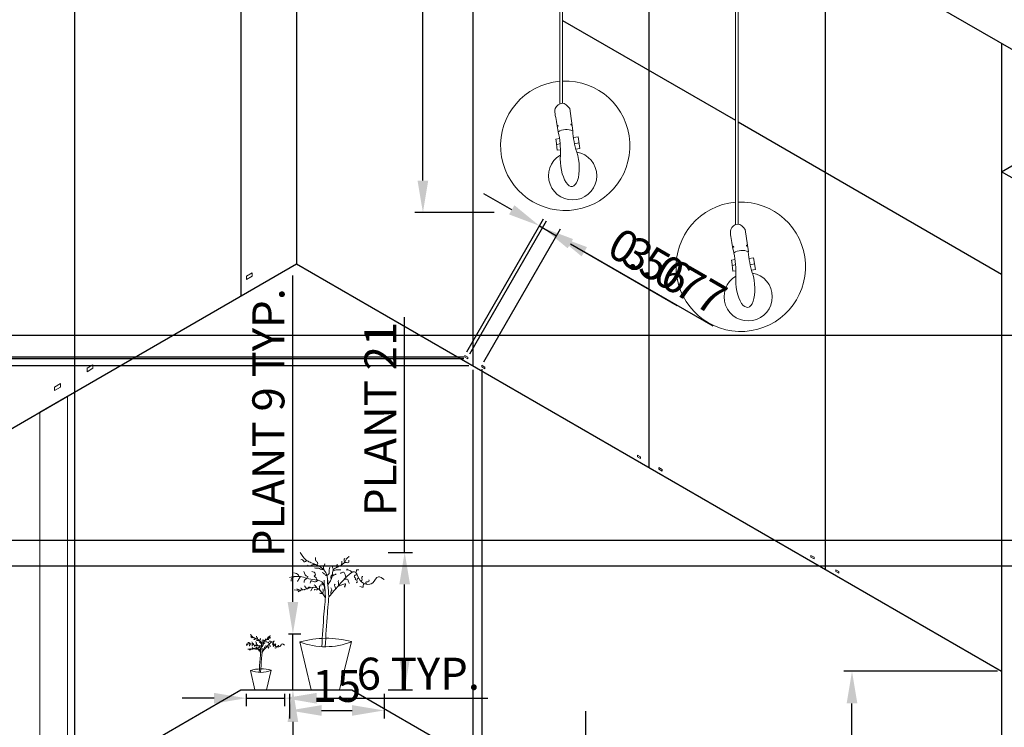
# Model space of a CAD drawing. Units: centimetres. Extents: x 2148 to 2649, y 4226 to 4785.
# Tile 4 of 6: x 2402 to 2555, y 4539 to 4649. Entities that reach past the tile are written whole.
import ezdxf

# ---------------------------------------------------------------- set-up
doc = ezdxf.new("R2010")
doc.units = ezdxf.units.CM
for name, color, linetype, lineweight in [('A-ANNO-DIMS', 63, 'Continuous', 18), ('A-ANNO-REFR', 8, 'Continuous', 13), ('A-FLOR-BSPL', 21, 'Continuous', 13), ('A-FLOR-CASE', 21, 'Continuous', 25), ('A-FLOR-CASE-HDW', 21, 'Continuous', 18), ('A-FLOR-CASE-TALL', 30, 'Continuous', 30), ('A-FLOR-CTOP', 21, 'Continuous', 25), ('E-LITE', 21, 'Continuous', 18), ('TREES', 80, 'Continuous', 13)]:
    doc.layers.add(name, color=color, linetype=linetype, lineweight=lineweight)
doc.styles.get("Standard").update_dxf_attribs({"font": 'arial.ttf'})
doc.dimstyles.new('ISO-25', dxfattribs={"dimtxt": 5, "dimasz": 5, "dimexe": 1.25, "dimexo": 0.625, "dimtad": 1, "dimdec": 1, "dimtxsty": 'Standard', "dimcen": 2.5, "dimadec": 0, "dimazin": 0, "dimtfac": 1, "dimtdec": 1, "dimtmove": 0, "dimatfit": 3, "dimfxl": 1, "dimarcsym": 0})

# ---------------------------------------------------------------- blocks, each defined once
blk = doc.blocks.new('*D1')
at = {"layer": 'A-ANNO-DIMS', "color": 0, "lineweight": -2, "transparency": 16777216}
for p, q in [((2409.99, 4699.79), (2406.08, 4706.55)), ((2255.15, 4617.96), (2402.38, 4702.96)), ((2254.1, 4609.79), (2250.2, 4616.55))]:
    blk.add_line(p, q, dxfattribs=at)
at = {"layer": 'A-ANNO-DIMS', "color": 0, "transparency": 16777216}
for points in [[(2401.96, 4703.69), (2402.8, 4702.24), (2406.71, 4705.46)], [(2254.74, 4618.69), (2255.57, 4617.24), (2250.82, 4615.46)]]:
    blk.add_solid(points, dxfattribs=at)
at = {"layer": 'Defpoints', "color": 0, "transparency": 16777216}
for p in [(2406.71, 4705.46), (2410.3, 4699.24), (2254.42, 4609.24)]:
    blk.add_point(p, dxfattribs=at)
at = {"layer": 'A-ANNO-DIMS', "color": 0, "transparency": 16777216, "insert": (2327.18, 4663.22), "char_height": 5, "attachment_point": 5, "rotation": 30}
blk.add_mtext('180', dxfattribs=at)
blk = doc.blocks.new('RECTANGLE')
for p, q in [((2256.66, 4502.65), (2260.99, 4505.15)), ((2260.99, 4443.76), (2260.99, 4505.15)), ((2256.66, 4502.65), (2256.66, 4441.26)), ((2256.66, 4441.26), (2260.99, 4443.76))]:
    blk.add_line(p, q)
blk = doc.blocks.new('*D5')
at = {"layer": 'A-ANNO-DIMS', "color": 0, "lineweight": -2, "transparency": 16777216}
for p, q in [((2435.97, 4714.79), (2427.84, 4728.87)), ((2193.77, 4592.29), (2424.13, 4725.29)), ((2196.95, 4576.79), (2188.81, 4590.87))]:
    blk.add_line(p, q, dxfattribs=at)
at = {"layer": 'A-ANNO-DIMS', "color": 0, "transparency": 16777216}
for points in [[(2423.72, 4726.01), (2424.55, 4724.57), (2428.46, 4727.79)], [(2193.35, 4593.01), (2194.19, 4591.57), (2189.44, 4589.79)]]:
    blk.add_solid(points, dxfattribs=at)
at = {"layer": 'Defpoints', "color": 0, "transparency": 16777216}
for p in [(2428.46, 4727.79), (2436.28, 4714.24), (2197.26, 4576.24)]:
    blk.add_point(p, dxfattribs=at)
at = {"layer": 'A-ANNO-DIMS', "color": 0, "transparency": 16777216, "insert": (2307.36, 4661.54), "char_height": 5, "attachment_point": 5, "rotation": 30}
blk.add_mtext('276', dxfattribs=at)
blk = doc.blocks.new('*D6')
at = {"layer": 'A-ANNO-DIMS', "color": 0, "lineweight": -2, "transparency": 16777216}
for p, q in [((2436.59, 4714.79), (2443.88, 4727.41)), ((2447.59, 4723.83), (2626.86, 4620.33)), ((2624.52, 4606.29), (2631.81, 4618.91))]:
    blk.add_line(p, q, dxfattribs=at)
at = {"layer": 'A-ANNO-DIMS', "color": 0, "transparency": 16777216}
for points in [[(2448.01, 4724.55), (2447.17, 4723.11), (2443.26, 4726.33)], [(2627.27, 4621.05), (2626.44, 4619.61), (2631.19, 4617.83)]]:
    blk.add_solid(points, dxfattribs=at)
at = {"layer": 'Defpoints', "color": 0, "transparency": 16777216}
for p in [(2436.28, 4714.24), (2631.19, 4617.83), (2624.21, 4605.74)]:
    blk.add_point(p, dxfattribs=at)
at = {"layer": 'A-ANNO-DIMS', "color": 0, "transparency": 16777216, "insert": (2538.79, 4674.79), "char_height": 5, "attachment_point": 5, "rotation": 330}
blk.add_mtext('217', dxfattribs=at)
blk = doc.blocks.new('TREE')
for p, q in [((2447.25, 4544.96), (2445.48, 4552.43)), ((2451.66, 4544.96), (2453.53, 4552.48))]:
    blk.add_line(p, q)
for centre, radius, start, end in [((2449.6, 4537.88), 15.12, 74.9103, 105.8034), ((2449.44, 4562.68), 11, 248.8663, 291.8473)]:
    blk.add_arc(centre, radius, start, end)
for points, knots in [([(2449.83, 4561.3), (2449.83, 4562.01), (2449.83, 4563.42), (2448.06, 4564.55), (2446.36, 4565.02), (2445.78, 4565.95), (2445.51, 4566.39)], [0, 0, 0, 0, 1.995568, 3.979762, 5.67782, 7.159715, 7.159715, 7.159715, 7.159715]), ([(2445.6, 4565.25), (2445.73, 4565.27), (2445.99, 4565.3), (2446.12, 4564.73), (2446.58, 4565.24), (2446.9, 4564.89), (2447.12, 4564.82), (2447.24, 4564.78)], [0, 0, 0, 0, 0.353698, 0.687974, 1.179754, 1.508828, 1.893119, 1.893119, 1.893119, 1.893119]), ([(2447.89, 4565.62), (2447.89, 4565.43), (2447.89, 4565.1), (2448.34, 4564.81), (2448.24, 4564.52), (2448.19, 4564.38)], [0, 0, 0, 0, 0.528266, 0.942976, 1.342243, 1.342243, 1.342243, 1.342243]), ([(2449.83, 4561.3), (2450.13, 4561.73), (2450.64, 4562.45), (2450.53, 4563.72), (2451.5, 4564.19), (2452.37, 4564.56), (2452.66, 4565.2), (2452.78, 4565.47)], [0, 0, 0, 0, 1.559218, 2.590263, 3.316916, 4.501885, 5.353772, 5.353772, 5.353772, 5.353772]), ([(2451.9, 4564.38), (2451.95, 4564.49), (2452.04, 4564.65), (2452.01, 4564.87), (2452.01, 4564.97), (2452.01, 4565)], [0, 0, 0, 0, 0.3358398, 0.5448262, 0.633178, 0.633178, 0.633178, 0.633178]), ([(2452.27, 4564.64), (2452.32, 4564.72), (2452.48, 4564.99), (2452.99, 4564.61), (2453.14, 4564.98), (2453.12, 4565.11), (2453.12, 4565.16)], [0, 0, 0, 0, 0.251714, 0.837833, 1.078551, 1.22335, 1.22335, 1.22335, 1.22335]), ([(2452.4, 4564.8), (2452.41, 4564.88), (2452.43, 4565.06), (2452.32, 4565.32), (2452.44, 4565.42), (2452.47, 4565.45)], [0, 0, 0, 0, 0.2491213, 0.5552893, 0.6860823, 0.6860823, 0.6860823, 0.6860823]), ([(2452.72, 4565.33), (2452.73, 4565.38), (2452.79, 4565.56), (2453.08, 4565.6), (2453.11, 4565.76), (2453.12, 4565.78)], [0, 0, 0, 0, 0.1482784, 0.5567745, 0.6230075, 0.6230075, 0.6230075, 0.6230075]), ([(2444.53, 4563.19), (2444.82, 4563.13), (2445.18, 4563.05), (2445.34, 4562.62), (2445.49, 4562.62), (2445.55, 4562.62)], [0, 0, 0, 0, 0.799643, 1.030684, 1.19755, 1.19755, 1.19755, 1.19755]), ([(2446.1, 4563.4), (2446.2, 4563.04), (2446.31, 4562.66), (2446.75, 4562.63), (2446.69, 4562.48), (2446.67, 4562.4), (2446.66, 4562.35)], [0, 0, 0, 0, 0.953341, 1.006749, 1.098323, 1.293043, 1.293043, 1.293043, 1.293043]), ([(2446.66, 4564.4), (2446.82, 4564.33), (2447.08, 4564.23), (2447.48, 4564.53), (2447.88, 4564.52), (2448.14, 4564.42), (2448.2, 4564.4)], [0, 0, 0, 0, 0.487977, 0.748703, 1.415993, 1.585236, 1.585236, 1.585236, 1.585236]), ([(2447.33, 4563.41), (2447.58, 4563.34), (2447.94, 4563.23), (2447.89, 4562.8), (2447.59, 4562.63), (2448.15, 4562.5), (2448.05, 4562.06), (2448.25, 4562.06), (2448.31, 4562.06)], [0, 0, 0, 0, 0.664801, 0.94436, 1.08206, 1.476917, 1.846316, 2.003009, 2.003009, 2.003009, 2.003009]), ([(2447.76, 4563.97), (2447.97, 4563.94), (2448.19, 4563.91), (2448.52, 4563.93), (2448.62, 4563.77), (2448.92, 4563.75), (2449.11, 4563.68), (2449.26, 4563.62)], [0, 0, 0, 0, 0.637067, 0.675943, 0.960411, 1.092541, 1.560471, 1.560471, 1.560471, 1.560471]), ([(2448.99, 4563.3), (2449.11, 4563.19), (2449.28, 4563.05), (2449.5, 4562.84), (2449.63, 4562.83), (2449.7, 4562.83)], [0, 0, 0, 0, 0.4862835, 0.6806136, 0.871086, 0.871086, 0.871086, 0.871086]), ([(2449.26, 4563.62), (2449.19, 4563.84), (2449.08, 4564.17), (2449.43, 4564.46), (2449.34, 4564.59), (2449.31, 4564.63)], [0, 0, 0, 0, 0.636403, 0.920765, 1.065556, 1.065556, 1.065556, 1.065556]), ([(2450.14, 4564.1), (2450.1, 4563.96), (2450, 4563.68), (2450.06, 4563.32), (2449.98, 4562.88), (2449.68, 4562.82), (2449.46, 4562.77)], [0, 0, 0, 0, 0.427172, 0.880416, 1.093996, 1.685063, 1.685063, 1.685063, 1.685063]), ([(2449.98, 4559.44), (2450.53, 4560.09), (2451.61, 4561.35), (2454.23, 4564.3), (2454.67, 4561.58), (2456.89, 4561.05), (2457.55, 4562.97), (2458.29, 4562.41), (2458.61, 4562.17)], [0, 0, 0, 0, 2.950259, 5.736815, 7.202351, 9.196187, 10.495572, 11.481506, 11.481506, 11.481506, 11.481506]), ([(2450.65, 4563.53), (2450.67, 4563.63), (2450.7, 4563.82), (2450.57, 4564.03), (2450.57, 4564.16), (2450.57, 4564.2)], [0, 0, 0, 0, 0.2987758, 0.5629986, 0.6917618, 0.6917618, 0.6917618, 0.6917618]), ([(2450.79, 4563.5), (2450.85, 4563.54), (2451.15, 4563.74), (2451.53, 4563.69), (2451.84, 4563.65)], [0, 0, 0, 0, 0.18742, 1.072841, 1.072841, 1.072841, 1.072841]), ([(2451.14, 4564.01), (2451.19, 4564.03), (2451.33, 4564.07), (2451.2, 4564.29), (2451.26, 4564.44), (2451.3, 4564.5), (2451.32, 4564.51)], [0, 0, 0, 0, 0.131224, 0.3928497, 0.5275017, 0.5966013, 0.5966013, 0.5966013, 0.5966013]), ([(2451.65, 4564.25), (2451.78, 4564.27), (2452.08, 4564.3), (2452.39, 4564.26), (2452.56, 4564.23)], [0, 0, 0, 0, 0.388997, 0.9136239, 0.9136239, 0.9136239, 0.9136239]), ([(2452.65, 4562.49), (2452.63, 4562.64), (2452.59, 4562.93), (2452.3, 4563.47), (2451.98, 4563.24), (2451.82, 4563.12)], [0, 0, 0, 0, 0.45479, 0.92627, 1.425708, 1.425708, 1.425708, 1.425708]), ([(2453.57, 4563.27), (2453.54, 4563.35), (2453.44, 4563.57), (2453.12, 4563.6), (2452.91, 4563.7), (2452.68, 4563.58), (2452.8, 4563.73), (2452.87, 4563.82)], [0, 0, 0, 0, 0.250514, 0.700182, 0.817059, 0.973893, 1.195588, 1.195588, 1.195588, 1.195588]), ([(2454.21, 4563.26), (2454.25, 4563.33), (2454.32, 4563.45), (2454.32, 4563.75), (2454.55, 4563.67), (2454.65, 4563.66), (2454.69, 4563.66)], [0, 0, 0, 0, 0.2405941, 0.4530054, 0.6562483, 0.7710751, 0.7710751, 0.7710751, 0.7710751]), ([(2449.39, 4560.41), (2449.32, 4560.98), (2449.16, 4562.11), (2447.09, 4562.07), (2445.55, 4562.82), (2444.32, 4562.59), (2443.85, 4562.5)], [0, 0, 0, 0, 1.50196, 2.979977, 5.268293, 6.6547, 6.6547, 6.6547, 6.6547]), ([(2444.83, 4562.66), (2444.5, 4562.55), (2444.06, 4562.4), (2444.1, 4562), (2444.11, 4561.9)], [0, 0, 0, 0, 0.86957, 1.154464, 1.154464, 1.154464, 1.154464]), ([(2445.55, 4562.62), (2445.49, 4562.52), (2445.4, 4562.36), (2445.26, 4562.12), (2445.18, 4561.91), (2445.06, 4561.89), (2445.04, 4561.89)], [0, 0, 0, 0, 0.3536471, 0.5448852, 0.8584322, 0.9118713, 0.9118713, 0.9118713, 0.9118713]), ([(2446.61, 4562.36), (2446.46, 4562.28), (2446.22, 4562.17), (2446.12, 4561.86), (2446.12, 4561.72), (2446.13, 4561.68)], [0, 0, 0, 0, 0.4813649, 0.7680471, 0.8975493, 0.8975493, 0.8975493, 0.8975493]), ([(2448.31, 4562.06), (2448.14, 4561.91), (2447.81, 4561.63), (2447.17, 4562.12), (2447.11, 4561.73), (2447.09, 4561.57)], [0, 0, 0, 0, 0.622646, 1.172708, 1.557766, 1.557766, 1.557766, 1.557766]), ([(2448.91, 4551.67), (2449, 4553.4), (2449.11, 4555.46), (2449.34, 4558.06), (2449.53, 4559.55), (2449.32, 4560.95), (2449.26, 4561.81), (2449.24, 4562.05)], [0, 0, 0, 0, 5.198408, 6.198659, 7.833196, 9.680738, 10.407711, 10.407711, 10.407711, 10.407711]), ([(2449.44, 4551.69), (2449.53, 4553.42), (2449.64, 4555.48), (2449.87, 4558.08), (2450.05, 4559.57), (2449.85, 4560.97), (2449.78, 4561.83), (2449.77, 4562.07)], [0, 0, 0, 0, 5.198408, 6.198659, 7.833196, 9.680738, 10.407711, 10.407711, 10.407711, 10.407711]), ([(2450.36, 4562.16), (2450.35, 4562.24), (2450.34, 4562.38), (2450.26, 4562.64), (2450.36, 4562.81), (2450.42, 4562.91)], [0, 0, 0, 0, 0.2419015, 0.4294094, 0.782934, 0.782934, 0.782934, 0.782934]), ([(2450.53, 4562.68), (2450.57, 4562.72), (2450.64, 4562.77), (2450.72, 4562.83), (2450.82, 4562.94), (2451.03, 4562.88), (2451.1, 4563), (2451.12, 4563.03)], [0, 0, 0, 0, 0.1839825, 0.2354423, 0.32084, 0.6015787, 0.715757, 0.715757, 0.715757, 0.715757]), ([(2451.4, 4561.1), (2452.09, 4561.38), (2452.96, 4561.74), (2452.35, 4561.06), (2452.51, 4561), (2452.56, 4560.99)], [0, 0, 0, 0, 1.194027, 1.500255, 1.630788, 1.630788, 1.630788, 1.630788]), ([(2451.48, 4561.19), (2451.51, 4561.32), (2451.55, 4561.5), (2451.46, 4561.77), (2451.47, 4561.92), (2451.48, 4562.03)], [0, 0, 0, 0, 0.3935209, 0.5296667, 0.851575, 0.851575, 0.851575, 0.851575]), ([(2452.32, 4562.14), (2452.6, 4562.23), (2453.1, 4562.38), (2452.98, 4561.72), (2453.18, 4561.6), (2453.24, 4561.57)], [0, 0, 0, 0, 0.657659, 1.152477, 1.342596, 1.342596, 1.342596, 1.342596]), ([(2454.41, 4562.99), (2454.17, 4562.89), (2453.74, 4562.72), (2454.23, 4562.34), (2454.12, 4562.17), (2454.1, 4562.14)], [0, 0, 0, 0, 0.56032, 1.008165, 1.121509, 1.121509, 1.121509, 1.121509]), ([(2454.61, 4562.45), (2454.46, 4562.3), (2454.24, 4562.09), (2454.49, 4561.73), (2454.33, 4561.66), (2454.26, 4561.63)], [0, 0, 0, 0, 0.537826, 0.7745438, 0.9749671, 0.9749671, 0.9749671, 0.9749671]), ([(2454.99, 4561.88), (2455.08, 4561.98), (2455.24, 4562.14), (2455.11, 4562.39), (2455.18, 4562.62), (2455.26, 4562.61), (2455.28, 4562.61)], [0, 0, 0, 0, 0.3499692, 0.6062162, 0.8045661, 0.8552851, 0.8552851, 0.8552851, 0.8552851]), ([(2455.86, 4561.43), (2455.78, 4561.56), (2455.6, 4561.89), (2456.32, 4561.69), (2456.26, 4561.99), (2456.23, 4562.1)], [0, 0, 0, 0, 0.333961, 0.823844, 1.08993, 1.08993, 1.08993, 1.08993]), ([(2449.45, 4559.33), (2448.92, 4560.14), (2448.1, 4561.4), (2446.22, 4560.44), (2445.17, 4560.51), (2444.56, 4560.54)], [0, 0, 0, 0, 2.40992, 3.739305, 5.578847, 5.578847, 5.578847, 5.578847]), ([(2445.01, 4560.71), (2445.17, 4560.62), (2445.37, 4560.5), (2445.62, 4560.51), (2445.68, 4560.52), (2445.69, 4560.52)], [0, 0, 0, 0, 0.5295015, 0.6942572, 0.7168035, 0.7168035, 0.7168035, 0.7168035]), ([(2445.19, 4560.23), (2445.23, 4560.26), (2445.34, 4560.32), (2445.53, 4560.36), (2445.62, 4560.47), (2445.66, 4560.52)], [0, 0, 0, 0, 0.157145, 0.3589113, 0.5662429, 0.5662429, 0.5662429, 0.5662429]), ([(2445.61, 4560.86), (2445.67, 4560.79), (2445.79, 4560.65), (2445.97, 4560.57), (2446.2, 4560.56), (2446.18, 4560.62), (2446.18, 4560.64)], [0, 0, 0, 0, 0.2483933, 0.5604364, 0.6736581, 0.7258462, 0.7258462, 0.7258462, 0.7258462]), ([(2446.22, 4561.18), (2446.38, 4560.89), (2446.62, 4560.47), (2446.85, 4561.06), (2447.05, 4560.94), (2447.15, 4560.88)], [0, 0, 0, 0, 0.64318, 0.967785, 1.239353, 1.239353, 1.239353, 1.239353]), ([(2447.66, 4560.97), (2447.54, 4560.94), (2447.32, 4560.88), (2447.34, 4560.55), (2447.21, 4560.45), (2447.15, 4560.41)], [0, 0, 0, 0, 0.333136, 0.6124023, 0.8146283, 0.8146283, 0.8146283, 0.8146283]), ([(2447.69, 4560.54), (2447.73, 4560.56), (2447.88, 4560.64), (2448.15, 4560.5), (2448.26, 4560.67), (2448.31, 4560.74)], [0, 0, 0, 0, 0.1577786, 0.4768013, 0.6980293, 0.6980293, 0.6980293, 0.6980293]), ([(2447.73, 4561.36), (2447.81, 4561.27), (2447.9, 4561.16), (2448.03, 4561), (2448.13, 4560.92), (2448.11, 4560.85), (2448.11, 4560.84)], [0, 0, 0, 0, 0.3534347, 0.4287436, 0.6404395, 0.6555943, 0.6555943, 0.6555943, 0.6555943]), ([(2448.68, 4560.4), (2448.6, 4560.54), (2448.48, 4560.74), (2448.57, 4561.03), (2448.51, 4561.14), (2448.48, 4561.19)], [0, 0, 0, 0, 0.4503193, 0.6632194, 0.8315566, 0.8315566, 0.8315566, 0.8315566]), ([(2449.25, 4561.22), (2449.08, 4561.38), (2448.82, 4561.62), (2448.7, 4561.25), (2448.74, 4561.15), (2448.74, 4561.13)], [0, 0, 0, 0, 0.4936671, 0.7765002, 0.8174683, 0.8174683, 0.8174683, 0.8174683]), ([(2449.05, 4559.93), (2449.07, 4560.03), (2449.1, 4560.2), (2449.14, 4560.46), (2449.08, 4560.61), (2449.04, 4560.7)], [0, 0, 0, 0, 0.3315498, 0.4956558, 0.7928621, 0.7928621, 0.7928621, 0.7928621]), ([(2450.35, 4559.88), (2450.3, 4560.05), (2450.24, 4560.27), (2450.53, 4560.53), (2450.4, 4560.73), (2450.3, 4560.87)], [0, 0, 0, 0, 0.457334, 0.622454, 1.040097, 1.040097, 1.040097, 1.040097]), ([(2451.04, 4560.68), (2451.04, 4560.78), (2451.05, 4560.99), (2450.8, 4561.22), (2450.91, 4561.38), (2450.96, 4561.45)], [0, 0, 0, 0, 0.308616, 0.5966018, 0.8330049, 0.8330049, 0.8330049, 0.8330049]), ([(2455.47, 4561.55), (2455.41, 4561.46), (2455.3, 4561.31), (2455.4, 4560.89), (2455.07, 4560.99), (2454.85, 4561.05)], [0, 0, 0, 0, 0.329722, 0.545126, 1.027082, 1.027082, 1.027082, 1.027082]), ([(2448.59, 4560), (2448.64, 4560.01), (2448.72, 4560.02), (2448.85, 4559.94), (2448.99, 4559.99), (2449.05, 4559.93), (2449.05, 4559.93)], [0, 0, 0, 0, 0.1309766, 0.2265734, 0.4607298, 0.4703086, 0.4703086, 0.4703086, 0.4703086])]:
    blk.add_open_spline(points, degree=3, knots=knots)
blk = doc.blocks.new('KNOB-ISO-R')
for p, q in [((0.49, 0.25), (0, 0.54)), ((0, 0.54), (0, 0.28)), ((0, 0.28), (0.49, 0)), ((0.49, 0), (0.49, 0.25))]:
    blk.add_line(p, q)
blk = doc.blocks.new('KNOB-ISO-L')
for p, q in [((0, 0.53), (0.92, 1.06)), ((0, 0), (0, 0.53)), ((0, 0), (0.92, 0.53)), ((0.92, 1.06), (0.92, 0.53))]:
    blk.add_line(p, q)
blk = doc.blocks.new('PENDANT-GLOBE')
for p, q in [((9.23, 16.63), (9.23, 76.94)), ((9.23, 16.63), (9.23, 76.94)), ((9.66, 16.72), (9.66, 76.98)), ((9.66, 16.72), (9.66, 76.98)), ((11.26, 12.41), (10.78, 15.92)), ((8.63, 11.11), (9.18, 11.2)), ((8.66, 10.87), (8.63, 11.11)), ((8.81, 9.4), (8.66, 10.87)), ((11.37, 11.36), (12.08, 11.47)), ((12.08, 11.47), (12.36, 9.65)), ((8.72, 10.24), (9.27, 10.46)), ((9.33, 9.46), (8.81, 9.4)), ((12.22, 10.56), (11.54, 10.41)), ((12.36, 9.65), (11.75, 9.55))]:
    blk.add_line(p, q)
for centre in [(8.89, 13.21), (11.04, 13.39)]:
    blk.add_circle(centre, 0.0802)
for centre, radius, start, end in [((9.99, 77.41), 1.68, 168.2535, 192.4899), ((8.39, 90.01), 12.26, 269.7881, 280.1017), ((9.16, 80.14), 3.21, 255.2356, 295.6813), ((9.7, 77.58), 0.908, 339.0828, 23.4705), ((10.08, 10.09), 10.09, 94.8735, 92.4088), ((10.25, 10.36), 2.28, 63.8319, 124.0685), ((25.64, 13.43), 14.43, 184.0611, 197.3987), ((-2.91, 9.3), 12.24, 356.9361, 13.9313), ((11.23, 5.41), 3.76, 120.6297, 80.001)]:
    blk.add_arc(centre, radius, start, end)
blk.add_ellipse((10.78, 7.32), major_axis=(0.37, -3.57), ratio=0.40259, start_param=4.289436, end_param=8.338162)
blk.add_open_spline([(8.53, 14.81), (8.46, 15.17), (8.29, 16.01), (9.68, 17.13), (10.41, 16.33), (10.78, 15.92)], degree=3, knots=[0, 0, 0, 0, 1.072444, 2.447575, 3.879684, 3.879684, 3.879684, 3.879684])
blk.add_open_spline([(8.97, 12.25), (8.82, 13.1), (8.68, 13.96), (8.53, 14.81)], degree=3)
blk = doc.blocks.new('*D26')
at = {"layer": 'A-ANNO-DIMS', "color": 0, "lineweight": -2, "transparency": 16777216}
for p, q in [((2464.67, 4697.64), (2464.67, 4785.41)), ((2475.78, 4697.64), (2463.42, 4697.64)), ((2464.67, 4624.36), (2464.67, 4692.64)), ((2475.78, 4619.36), (2463.42, 4619.36))]:
    blk.add_line(p, q, dxfattribs=at)
at = {"layer": 'A-ANNO-DIMS', "color": 0, "transparency": 16777216}
for points in [[(2463.83, 4692.64), (2465.5, 4692.64), (2464.67, 4697.64)], [(2463.83, 4624.36), (2465.5, 4624.36), (2464.67, 4619.36)]]:
    blk.add_solid(points, dxfattribs=at)
at = {"layer": 'Defpoints', "color": 0, "transparency": 16777216}
for p in [(2464.67, 4697.64), (2476.41, 4697.64), (2476.41, 4619.36)]:
    blk.add_point(p, dxfattribs=at)
at = {"layer": 'A-ANNO-DIMS', "color": 0, "transparency": 16777216, "insert": (2461.45, 4744.03), "char_height": 5, "attachment_point": 5, "rotation": 90}
blk.add_mtext('PENDANT DROP 78 TYP.', dxfattribs=at)
blk = doc.blocks.new('*D29')
at = {"layer": 'A-ANNO-DIMS', "color": 0, "lineweight": -2, "transparency": 16777216}
for p, q in [((2490.09, 4536.62), (2490.09, 4541.62)), ((2488.18, 4531.62), (2491.34, 4531.62)), ((2490.09, 4521.87), (2490.09, 4531.62)), ((2488.18, 4521.87), (2491.34, 4521.87)), ((2490.09, 4516.87), (2490.09, 4511.87))]:
    blk.add_line(p, q, dxfattribs=at)
at = {"layer": 'A-ANNO-DIMS', "color": 0, "transparency": 16777216}
for points in [[(2489.26, 4536.62), (2490.92, 4536.62), (2490.09, 4531.62)], [(2489.26, 4516.87), (2490.92, 4516.87), (2490.09, 4521.87)]]:
    blk.add_solid(points, dxfattribs=at)
at = {"layer": 'Defpoints', "color": 0, "transparency": 16777216}
for p in [(2487.56, 4531.62), (2490.09, 4531.62), (2487.56, 4521.87)]:
    blk.add_point(p, dxfattribs=at)
at = {"layer": 'A-ANNO-DIMS', "color": 0, "transparency": 16777216, "insert": (2486.91, 4526.75), "char_height": 5, "attachment_point": 5, "rotation": 90}
blk.add_mtext('10', dxfattribs=at)
blk = doc.blocks.new('*D36')
at = {"layer": 'A-ANNO-DIMS', "color": 0, "lineweight": -2, "transparency": 16777216}
for p, q in [((2461.82, 4566.39), (2461.82, 4603.04)), ((2459.24, 4566.39), (2463.07, 4566.39)), ((2461.82, 4549.96), (2461.82, 4561.39)), ((2459.24, 4544.96), (2463.07, 4544.96))]:
    blk.add_line(p, q, dxfattribs=at)
at = {"layer": 'A-ANNO-DIMS', "color": 0, "transparency": 16777216}
for points in [[(2460.99, 4561.39), (2462.66, 4561.39), (2461.82, 4566.39)], [(2460.99, 4549.96), (2462.66, 4549.96), (2461.82, 4544.96)]]:
    blk.add_solid(points, dxfattribs=at)
at = {"layer": 'Defpoints', "color": 0, "transparency": 16777216}
for p in [(2458.61, 4566.39), (2461.82, 4566.39), (2458.61, 4544.96)]:
    blk.add_point(p, dxfattribs=at)
at = {"layer": 'A-ANNO-DIMS', "color": 0, "transparency": 16777216, "insert": (2458.69, 4587.21), "char_height": 5, "attachment_point": 5, "rotation": 90}
blk.add_mtext('PLANT 21', dxfattribs=at)
blk = doc.blocks.new('*D37')
at = {"layer": 'A-ANNO-DIMS', "color": 0, "lineweight": -2, "transparency": 16777216}
for p, q in [((2443.85, 4544.34), (2443.85, 4540.5)), ((2458.61, 4544.34), (2458.61, 4540.5)), ((2448.85, 4541.75), (2453.61, 4541.75))]:
    blk.add_line(p, q, dxfattribs=at)
at = {"layer": 'A-ANNO-DIMS', "color": 0, "transparency": 16777216}
for points in [[(2448.85, 4542.58), (2448.85, 4540.92), (2443.85, 4541.75)], [(2453.61, 4542.58), (2453.61, 4540.92), (2458.61, 4541.75)]]:
    blk.add_solid(points, dxfattribs=at)
at = {"layer": 'Defpoints', "color": 0, "transparency": 16777216}
for p in [(2443.85, 4544.96), (2458.61, 4544.96), (2458.61, 4541.75)]:
    blk.add_point(p, dxfattribs=at)
at = {"layer": 'A-ANNO-DIMS', "color": 0, "transparency": 16777216, "insert": (2451.23, 4544.93), "char_height": 5, "attachment_point": 5}
blk.add_mtext('15', dxfattribs=at)
blk = doc.blocks.new('*D38')
at = {"layer": 'A-ANNO-DIMS', "color": 0, "lineweight": -2, "transparency": 16777216}
for p, q in [((2444.39, 4558.67), (2444.39, 4609.58)), ((2443.71, 4553.67), (2445.64, 4553.67)), ((2444.39, 4544.96), (2444.39, 4553.67)), ((2443.71, 4544.96), (2445.64, 4544.96)), ((2444.39, 4539.96), (2444.39, 4534.96))]:
    blk.add_line(p, q, dxfattribs=at)
at = {"layer": 'A-ANNO-DIMS', "color": 0, "transparency": 16777216}
for points in [[(2443.56, 4558.67), (2445.22, 4558.67), (2444.39, 4553.67)], [(2443.56, 4539.96), (2445.22, 4539.96), (2444.39, 4544.96)]]:
    blk.add_solid(points, dxfattribs=at)
at = {"layer": 'Defpoints', "color": 0, "transparency": 16777216}
for p in [(2443.09, 4553.67), (2444.39, 4553.67), (2443.09, 4544.96)]:
    blk.add_point(p, dxfattribs=at)
at = {"layer": 'A-ANNO-DIMS', "color": 0, "transparency": 16777216, "insert": (2441.21, 4586.62), "char_height": 5, "attachment_point": 5, "rotation": 90}
blk.add_mtext('PLANT 9 TYP.', dxfattribs=at)
blk = doc.blocks.new('*D39')
at = {"layer": 'A-ANNO-DIMS', "color": 0, "lineweight": -2, "transparency": 16777216}
for p, q in [((2432.09, 4543.66), (2427.09, 4543.66)), ((2437.09, 4544.34), (2437.09, 4542.41)), ((2437.09, 4543.66), (2443.09, 4543.66)), ((2443.09, 4544.34), (2443.09, 4542.41)), ((2448.09, 4543.66), (2474.82, 4543.66))]:
    blk.add_line(p, q, dxfattribs=at)
at = {"layer": 'A-ANNO-DIMS', "color": 0, "transparency": 16777216}
for points in [[(2432.09, 4544.49), (2432.09, 4542.82), (2437.09, 4543.66)], [(2448.09, 4544.49), (2448.09, 4542.82), (2443.09, 4543.66)]]:
    blk.add_solid(points, dxfattribs=at)
at = {"layer": 'Defpoints', "color": 0, "transparency": 16777216}
for p in [(2437.09, 4544.96), (2443.09, 4544.96), (2443.09, 4543.66)]:
    blk.add_point(p, dxfattribs=at)
at = {"layer": 'A-ANNO-DIMS', "color": 0, "transparency": 16777216, "insert": (2463.95, 4546.83), "char_height": 5, "attachment_point": 5}
blk.add_mtext('6 TYP.', dxfattribs=at)
blk = doc.blocks.new('*D42')
at = {"layer": 'A-ANNO-DIMS', "color": 0, "lineweight": -2, "transparency": 16777216}
for p, q in [((2305.27, 4600.28), (2648.78, 4600.28)), ((2647.53, 4595.28), (2647.53, 4573.32)), ((2305.27, 4568.32), (2648.78, 4568.32))]:
    blk.add_line(p, q, dxfattribs=at)
at = {"layer": 'A-ANNO-DIMS', "color": 0, "transparency": 16777216}
for points in [[(2646.7, 4595.28), (2648.37, 4595.28), (2647.53, 4600.28)], [(2646.7, 4573.32), (2648.37, 4573.32), (2647.53, 4568.32)]]:
    blk.add_solid(points, dxfattribs=at)
at = {"layer": 'Defpoints', "color": 0, "transparency": 16777216}
for p in [(2304.65, 4600.28), (2304.65, 4568.32), (2647.53, 4568.32)]:
    blk.add_point(p, dxfattribs=at)
at = {"layer": 'A-ANNO-DIMS', "color": 0, "transparency": 16777216, "insert": (2644.35, 4584.3), "char_height": 5, "attachment_point": 5, "rotation": 90}
blk.add_mtext('31.96', dxfattribs=at)
blk = doc.blocks.new('*D43')
at = {"layer": 'A-ANNO-DIMS', "color": 0, "lineweight": -2, "transparency": 16777216}
for p, q in [((2647.53, 4573.32), (2647.53, 4578.32)), ((2305.27, 4568.32), (2648.78, 4568.32)), ((2647.53, 4568.32), (2647.53, 4564.32)), ((2305.27, 4564.32), (2648.78, 4564.32)), ((2647.53, 4559.32), (2647.53, 4549.61))]:
    blk.add_line(p, q, dxfattribs=at)
at = {"layer": 'A-ANNO-DIMS', "color": 0, "transparency": 16777216}
for points in [[(2646.7, 4573.32), (2648.37, 4573.32), (2647.53, 4568.32)], [(2646.7, 4559.32), (2648.37, 4559.32), (2647.53, 4564.32)]]:
    blk.add_solid(points, dxfattribs=at)
at = {"layer": 'Defpoints', "color": 0, "transparency": 16777216}
for p in [(2304.65, 4568.32), (2304.65, 4564.32), (2647.53, 4564.32)]:
    blk.add_point(p, dxfattribs=at)
at = {"layer": 'A-ANNO-DIMS', "color": 0, "transparency": 16777216, "insert": (2644.41, 4551.97), "char_height": 5, "attachment_point": 5, "rotation": 90}
blk.add_mtext('4', dxfattribs=at)
blk = doc.blocks.new('*D44')
at = {"layer": 'A-ANNO-DIMS', "color": 0, "lineweight": -2, "transparency": 16777216}
for p, q in [((2305.27, 4564.32), (2648.78, 4564.32)), ((2647.53, 4559.32), (2647.53, 4535.36)), ((2305.27, 4530.36), (2648.78, 4530.36))]:
    blk.add_line(p, q, dxfattribs=at)
at = {"layer": 'A-ANNO-DIMS', "color": 0, "transparency": 16777216}
for points in [[(2646.7, 4559.32), (2648.37, 4559.32), (2647.53, 4564.32)], [(2646.7, 4535.36), (2648.37, 4535.36), (2647.53, 4530.36)]]:
    blk.add_solid(points, dxfattribs=at)
at = {"layer": 'Defpoints', "color": 0, "transparency": 16777216}
for p in [(2304.65, 4564.32), (2304.65, 4530.36), (2647.53, 4530.36)]:
    blk.add_point(p, dxfattribs=at)
at = {"layer": 'A-ANNO-DIMS', "color": 0, "transparency": 16777216, "insert": (2644.35, 4547.34), "char_height": 5, "attachment_point": 5, "rotation": 90}
blk.add_mtext('33.96', dxfattribs=at)
blk = doc.blocks.new('*D45')
at = {"layer": 'A-ANNO-DIMS', "color": 0, "lineweight": -2, "transparency": 16777216}
for p, q in [((2478.52, 4619.8), (2474.19, 4622.3)), ((2471.5, 4597.64), (2483.48, 4618.38)), ((2471.99, 4597.36), (2483.97, 4618.1)), ((2482.85, 4617.3), (2483.34, 4617.02)), ((2487.67, 4614.52), (2504.33, 4604.9))]:
    blk.add_line(p, q, dxfattribs=at)
at = {"layer": 'A-ANNO-DIMS', "color": 0, "transparency": 16777216}
for points in [[(2478.94, 4620.52), (2478.11, 4619.08), (2482.85, 4617.3)], [(2488.09, 4615.24), (2487.25, 4613.8), (2483.34, 4617.02)]]:
    blk.add_solid(points, dxfattribs=at)
at = {"layer": 'Defpoints', "color": 0, "transparency": 16777216}
for p in [(2483.34, 4617.02), (2471.19, 4597.1), (2471.68, 4596.82)]:
    blk.add_point(p, dxfattribs=at)
at = {"layer": 'A-ANNO-DIMS', "color": 0, "transparency": 16777216, "insert": (2499.75, 4611.21), "char_height": 5, "attachment_point": 5, "rotation": 330}
blk.add_mtext('0.56', dxfattribs=at)
blk = doc.blocks.new('*D46')
at = {"layer": 'A-ANNO-DIMS', "color": 0, "lineweight": -2, "transparency": 16777216}
for p, q in [((2154.93, 4601.82), (2154.93, 4606.82)), ((2471.05, 4596.82), (2153.68, 4596.82)), ((2471.05, 4596.57), (2153.68, 4596.57)), ((2154.93, 4596.82), (2154.93, 4596.57)), ((2154.93, 4591.57), (2154.93, 4572.29))]:
    blk.add_line(p, q, dxfattribs=at)
at = {"layer": 'A-ANNO-DIMS', "color": 0, "transparency": 16777216}
for points in [[(2154.1, 4601.82), (2155.77, 4601.82), (2154.93, 4596.82)], [(2154.1, 4591.57), (2155.77, 4591.57), (2154.93, 4596.57)]]:
    blk.add_solid(points, dxfattribs=at)
at = {"layer": 'Defpoints', "color": 0, "transparency": 16777216}
for p in [(2154.93, 4596.57), (2471.68, 4596.82), (2471.68, 4596.57)]:
    blk.add_point(p, dxfattribs=at)
at = {"layer": 'A-ANNO-DIMS', "color": 0, "transparency": 16777216, "insert": (2151.75, 4579.43), "char_height": 5, "attachment_point": 5, "rotation": 90}
blk.add_mtext('0.25', dxfattribs=at)
blk = doc.blocks.new('*D47')
at = {"layer": 'A-ANNO-DIMS', "color": 0, "lineweight": -2, "transparency": 16777216}
for p, q in [((2478.52, 4619.8), (2474.19, 4622.3)), ((2471.5, 4597.64), (2483.48, 4618.38)), ((2482.85, 4617.3), (2485.52, 4615.76)), ((2474.17, 4596.1), (2486.14, 4616.85)), ((2489.85, 4613.26), (2509.87, 4601.7))]:
    blk.add_line(p, q, dxfattribs=at)
at = {"layer": 'A-ANNO-DIMS', "color": 0, "transparency": 16777216}
for points in [[(2478.94, 4620.52), (2478.11, 4619.08), (2482.85, 4617.3)], [(2490.27, 4613.99), (2489.43, 4612.54), (2485.52, 4615.76)]]:
    blk.add_solid(points, dxfattribs=at)
at = {"layer": 'Defpoints', "color": 0, "transparency": 16777216}
for p in [(2485.52, 4615.76), (2471.19, 4597.1), (2473.86, 4595.56)]:
    blk.add_point(p, dxfattribs=at)
at = {"layer": 'A-ANNO-DIMS', "color": 0, "transparency": 16777216, "insert": (2503.61, 4608.99), "char_height": 5, "attachment_point": 5, "rotation": 330}
blk.add_mtext('3.077', dxfattribs=at)
blk = doc.blocks.new('*D48')
at = {"layer": 'A-ANNO-DIMS', "color": 0, "lineweight": -2, "transparency": 16777216}
for p, q in [((2472.44, 4594.86), (2472.44, 4242.8)), ((2473.86, 4594.94), (2473.86, 4242.8)), ((2467.44, 4244.05), (2462.44, 4244.05)), ((2472.44, 4244.05), (2473.86, 4244.05)), ((2478.86, 4244.05), (2497.57, 4244.05))]:
    blk.add_line(p, q, dxfattribs=at)
at = {"layer": 'A-ANNO-DIMS', "color": 0, "transparency": 16777216}
for points in [[(2467.44, 4244.88), (2467.44, 4243.21), (2472.44, 4244.05)], [(2478.86, 4244.88), (2478.86, 4243.21), (2473.86, 4244.05)]]:
    blk.add_solid(points, dxfattribs=at)
at = {"layer": 'Defpoints', "color": 0, "transparency": 16777216}
for p in [(2472.44, 4595.48), (2473.86, 4595.56), (2473.86, 4244.05)]:
    blk.add_point(p, dxfattribs=at)
at = {"layer": 'A-ANNO-DIMS', "color": 0, "transparency": 16777216, "insert": (2490.71, 4247.18), "char_height": 5, "attachment_point": 5}
blk.add_mtext('1.42', dxfattribs=at)
blk = doc.blocks.new('*D49')
at = {"layer": 'A-ANNO-DIMS', "color": 0, "lineweight": -2, "transparency": 16777216}
for p, q in [((2154.93, 4601.85), (2154.93, 4620.61)), ((2470.57, 4596.85), (2153.68, 4596.85)), ((2471.81, 4595.48), (2153.68, 4595.48)), ((2154.93, 4595.48), (2154.93, 4596.85)), ((2154.93, 4590.48), (2154.93, 4585.48))]:
    blk.add_line(p, q, dxfattribs=at)
at = {"layer": 'A-ANNO-DIMS', "color": 0, "transparency": 16777216}
for points in [[(2154.1, 4601.85), (2155.77, 4601.85), (2154.93, 4596.85)], [(2154.1, 4590.48), (2155.77, 4590.48), (2154.93, 4595.48)]]:
    blk.add_solid(points, dxfattribs=at)
at = {"layer": 'Defpoints', "color": 0, "transparency": 16777216}
for p in [(2154.93, 4596.85), (2471.19, 4596.85), (2472.44, 4595.48)]:
    blk.add_point(p, dxfattribs=at)
at = {"layer": 'A-ANNO-DIMS', "color": 0, "transparency": 16777216, "insert": (2151.75, 4613.73), "char_height": 5, "attachment_point": 5, "rotation": 90}
blk.add_mtext('1.37', dxfattribs=at)
blk = doc.blocks.new('*D50')
at = {"layer": 'A-ANNO-DIMS', "color": 0, "lineweight": -2, "transparency": 16777216}
for p, q in [((2178.26, 4588.31), (2178.26, 4738.82)), ((2624.21, 4606.37), (2624.21, 4738.82)), ((2183.26, 4737.57), (2619.21, 4737.57))]:
    blk.add_line(p, q, dxfattribs=at)
at = {"layer": 'A-ANNO-DIMS', "color": 0, "transparency": 16777216}
for points in [[(2183.26, 4738.4), (2183.26, 4736.74), (2178.26, 4737.57)], [(2619.21, 4738.4), (2619.21, 4736.74), (2624.21, 4737.57)]]:
    blk.add_solid(points, dxfattribs=at)
at = {"layer": 'Defpoints', "color": 0, "transparency": 16777216}
for p in [(2624.21, 4737.57), (2624.21, 4605.74), (2178.26, 4587.69)]:
    blk.add_point(p, dxfattribs=at)
at = {"layer": 'A-ANNO-DIMS', "color": 0, "transparency": 16777216, "insert": (2401.23, 4740.75), "char_height": 5, "attachment_point": 5}
blk.add_mtext('445.95', dxfattribs=at)
blk = doc.blocks.new('*D51')
at = {"layer": 'A-ANNO-DIMS', "color": 0, "lineweight": -2, "transparency": 16777216}
for p, q in [((2436.91, 4714.24), (2648.78, 4714.24)), ((2647.53, 4272.37), (2647.53, 4709.24)), ((2409.81, 4267.37), (2648.78, 4267.37))]:
    blk.add_line(p, q, dxfattribs=at)
at = {"layer": 'A-ANNO-DIMS', "color": 0, "transparency": 16777216}
for points in [[(2646.7, 4709.24), (2648.37, 4709.24), (2647.53, 4714.24)], [(2646.7, 4272.37), (2648.37, 4272.37), (2647.53, 4267.37)]]:
    blk.add_solid(points, dxfattribs=at)
at = {"layer": 'Defpoints', "color": 0, "transparency": 16777216}
for p in [(2436.28, 4714.24), (2647.53, 4714.24), (2409.18, 4267.37)]:
    blk.add_point(p, dxfattribs=at)
at = {"layer": 'A-ANNO-DIMS', "color": 0, "transparency": 16777216, "insert": (2644.36, 4490.81), "char_height": 5, "attachment_point": 5, "rotation": 90}
blk.add_mtext('446.9', dxfattribs=at)
blk = doc.blocks.new('*D59')
at = {"layer": 'A-ANNO-DIMS', "color": 0, "lineweight": -2, "transparency": 16777216}
for p, q in [((2554.3, 4547.86), (2530.35, 4547.86)), ((2531.6, 4491.46), (2531.6, 4542.86)), ((2554.3, 4486.46), (2530.35, 4486.46))]:
    blk.add_line(p, q, dxfattribs=at)
at = {"layer": 'A-ANNO-DIMS', "color": 0, "transparency": 16777216}
for points in [[(2530.77, 4542.86), (2532.43, 4542.86), (2531.6, 4547.86)], [(2530.77, 4491.46), (2532.43, 4491.46), (2531.6, 4486.46)]]:
    blk.add_solid(points, dxfattribs=at)
at = {"layer": 'Defpoints', "color": 0, "transparency": 16777216}
for p in [(2531.6, 4547.86), (2554.93, 4547.86), (2554.93, 4486.46)]:
    blk.add_point(p, dxfattribs=at)
at = {"layer": 'A-ANNO-DIMS', "color": 0, "transparency": 16777216, "insert": (2528.42, 4517.16), "char_height": 5, "attachment_point": 5, "rotation": 90}
blk.add_mtext('61.4', dxfattribs=at)

msp = doc.modelspace()

# ---------------------------------------------------------------- linework, layer by layer
at = {"layer": 'A-ANNO-REFR'}
for p in [(2499.934, 4623.3597), (2527.4303, 4607.4847)]:
    msp.add_point(p, dxfattribs=at)
at = {"layer": 'A-FLOR-CASE'}
for p, q in [((2436.2812, 4714.2447), (2436.2812, 4606.357)), ((2444.9414, 4709.2447), (2444.9414, 4611.357)), ((2410.3004, 4699.2447), (2410.3004, 4529.9623)), ((2472.4377, 4693.3697), (2472.4377, 4595.482)), ((2499.934, 4677.4947), (2499.934, 4579.607)), ((2513.8379, 4669.4674), (2572.2471, 4635.7447)), ((2527.4303, 4661.6197), (2527.4303, 4563.732)), ((2486.4537, 4649.3151), (2513.4048, 4633.7548)), ((2513.8379, 4633.5048), (2554.9266, 4609.7822)), ((2410.3004, 4591.357), (2444.9414, 4611.357)), ((2444.9414, 4611.357), (2554.9266, 4547.857)), ((2362.545, 4563.7854), (2410.3004, 4591.357))]:
    msp.add_line(p, q, dxfattribs=at)
at = {"layer": 'A-FLOR-CASE-TALL'}
for p, q in [((2554.9266, 4645.7447), (2554.9266, 4369.7671)), ((2554.9266, 4625.7447), (2572.2471, 4635.7447)), ((2606.8882, 4595.7447), (2554.9266, 4625.7447))]:
    msp.add_line(p, q, dxfattribs=at)
at = {"layer": 'A-FLOR-CTOP'}
for p, q in [((2409.2302, 4529.3444), (2436.2812, 4544.9623)), ((2436.2812, 4544.9623), (2453.6017, 4544.9623)), ((2453.6017, 4544.9623), (2532.1733, 4499.5989))]:
    msp.add_line(p, q, dxfattribs=at)

# ---------------------------------------------------------------- block references
at = {"layer": 'A-FLOR-BSPL'}
msp.add_blockref('RECTANGLE', (148.243, 85.5881), dxfattribs=at)
at = {"layer": 'A-FLOR-CASE-HDW'}
for name, p in [('KNOB-ISO-L', (2437.135, 4608.912)), ('KNOB-ISO-R', (2471.1913, 4596.5665)), ('KNOB-ISO-L', (2412.2806, 4594.5623)), ('KNOB-ISO-R', (2473.856, 4595.028)), ('KNOB-ISO-L', (2407.2179, 4591.6394)), ('KNOB-ISO-R', (2498.1223, 4581.0179)), ('KNOB-ISO-R', (2501.4953, 4579.0705)), ('KNOB-ISO-R', (2525.1899, 4565.3904)), ('KNOB-ISO-R', (2529.0721, 4563.149))]:
    msp.add_blockref(name, p, dxfattribs=at)
at = {"layer": 'E-LITE'}
for p in [(2476.793, 4619.696), (2504.1772, 4600.8355)]:
    msp.add_blockref('PENDANT-GLOBE', p, dxfattribs=at)
at = {"layer": 'TREES'}
msp.add_blockref('TREE', (0, 0), dxfattribs=at)
at = {"layer": 'TREES', "xscale": 0.4062539037300824, "yscale": 0.4062539037300824, "zscale": 0.4062539037300824}
msp.add_blockref('TREE', (1444.2651, 2698.5536), dxfattribs=at)

# ---------------------------------------------------------------- dimensions: what is measured, and where the dimension line sits
at = {"layer": 'A-ANNO-DIMS'}
for base, p1, p2, text, picture, middle in [((2464.6668, 4697.6363), (2476.4076, 4619.3648), (2476.4076, 4697.6363), 'PENDANT DROP <> TYP.', '*D26', (2461.4549, 4744.0253)), ((2444.391, 4553.6666), (2443.0854, 4544.9623), (2443.0854, 4553.6666), 'PLANT <> TYP.', '*D38', (2441.2132, 4586.621)), ((2461.8248, 4566.3881), (2458.6109, 4544.9623), (2458.6109, 4566.3881), 'PLANT <>', '*D36', (2458.6878, 4587.2143))]:
    dim = msp.add_linear_dim(base=base, p1=p1, p2=p2, angle=90, text=text, dimstyle='ISO-25', override={"dimdec": 0, "dimlfac": 1, "dimrnd": 0, "dimzin": 0, "dimdsep": 46, "dimlunit": 2}, dxfattribs=at)
    dim.commit()
    dim.dimension.update_dxf_attribs({"geometry": picture, "text_midpoint": middle})
for base, p1, p2, override, picture, middle in [((2624.2087, 4737.5697), (2178.2568, 4587.6856), (2624.2087, 4605.7447), {"dimdec": 2, "dimlfac": 1, "dimrnd": 0, "dimzin": 0, "dimdsep": 46, "dimlunit": 2}, '*D50', (2401.2328, 4740.7476)), ((2473.8561, 4244.0481), (2472.4377, 4595.482), (2473.8561, 4595.5637), {"dimdec": 2, "dimlfac": 1, "dimrnd": 0, "dimzin": 0, "dimdsep": 46, "dimlunit": 2}, '*D48', (2490.714, 4247.1833)), ((2458.6109, 4541.7484), (2443.8517, 4544.9623), (2458.6109, 4544.9623), {"dimdec": 0, "dimlfac": 1, "dimrnd": 0, "dimzin": 0, "dimdsep": 46, "dimlunit": 2}, '*D37', (2451.2313, 4544.9263))]:
    dim = msp.add_linear_dim(base=base, p1=p1, p2=p2, dimstyle='ISO-25', override=override, dxfattribs=at)
    dim.commit()
    dim.dimension.update_dxf_attribs({"geometry": picture, "text_midpoint": middle})
for p1, p2, distance, picture, middle in [((2197.2581, 4576.2447), (2436.2812, 4714.2447), 15.6376, '*D5', (2307.3619, 4661.5394)), ((2436.2812, 4714.2447), (2624.2087, 4605.7447), 13.9546, '*D6', (2538.7898, 4674.795)), ((2254.4158, 4609.2447), (2410.3004, 4699.2447), 7.1825, '*D1', (2327.1779, 4663.217))]:
    dim = msp.add_aligned_dim(p1=p1, p2=p2, distance=distance, dimstyle='ISO-25', override={"dimclrd": 0, "dimclre": 0, "dimclrt": 0}, dxfattribs=at)
    dim.commit()
    dim.dimension.update_dxf_attribs({"geometry": picture, "text_midpoint": middle})
for base, p1, p2, angle, override, picture, middle in [((2647.5337, 4714.2447), (2409.1829, 4267.3731), (2436.2812, 4714.2447), 90, {"dimdec": 1, "dimlfac": 1, "dimrnd": 0, "dimzin": 0, "dimdsep": 46, "dimlunit": 2}, '*D51', (2644.3558, 4490.8089)), ((2483.3404, 4617.0213), (2471.1914, 4597.1021), (2471.6779, 4596.8213), 330, {"dimdec": 2, "dimlfac": 1, "dimrnd": 0, "dimzin": 0, "dimdsep": 46, "dimlunit": 2}, '*D45', (2499.7532, 4611.2149)), ((2485.5186, 4615.7637), (2471.1914, 4597.1021), (2473.8561, 4595.5637), 330, {"dimdec": 3, "dimlfac": 1, "dimrnd": 0, "dimzin": 0, "dimdsep": 46, "dimlunit": 2}, '*D47', (2503.6144, 4608.9876)), ((2154.9318, 4596.8477), (2472.4377, 4595.482), (2471.1914, 4596.8477), 90, {"dimdec": 2, "dimlfac": 1, "dimrnd": 0, "dimzin": 0, "dimdsep": 46, "dimlunit": 2}, '*D49', (2151.7523, 4613.7312)), ((2154.9318, 4596.5668), (2471.6779, 4596.8213), (2471.6779, 4596.5668), 90, {"dimdec": 2, "dimlfac": 1, "dimrnd": 0, "dimzin": 0, "dimdsep": 46, "dimlunit": 2}, '*D46', (2151.754, 4579.4292)), ((2647.5337, 4568.3196), (2304.6453, 4600.2822), (2304.6453, 4568.3196), 90, {"dimdec": 2, "dimlfac": 1, "dimrnd": 0, "dimzin": 0, "dimdsep": 46, "dimlunit": 2}, '*D42', (2644.3541, 4584.3009)), ((2647.5337, 4564.3196), (2304.6453, 4568.3196), (2304.6453, 4564.3196), 90, {"dimdec": 0, "dimlfac": 1, "dimrnd": 0, "dimzin": 0, "dimdsep": 46, "dimlunit": 2}, '*D43', (2644.4087, 4551.9654)), ((2647.5337, 4530.357), (2304.6453, 4564.3196), (2304.6453, 4530.357), 90, {"dimdec": 2, "dimlfac": 1, "dimrnd": 0, "dimzin": 0, "dimdsep": 46, "dimlunit": 2}, '*D44', (2644.3541, 4547.3383)), ((2531.6016, 4547.857), (2554.9266, 4486.4623), (2554.9266, 4547.857), 90, {"dimdec": 1, "dimlfac": 1, "dimrnd": 0, "dimzin": 0, "dimdsep": 46, "dimlunit": 2}, '*D59', (2528.4238, 4517.1596)), ((2490.0907, 4531.6197), (2487.5585, 4521.8734), (2487.5585, 4531.6197), 90, {"dimdec": 0, "dimlfac": 1, "dimrnd": 0, "dimzin": 0, "dimdsep": 46, "dimlunit": 2}, '*D29', (2486.9129, 4526.7466))]:
    dim = msp.add_linear_dim(base=base, p1=p1, p2=p2, angle=angle, dimstyle='ISO-25', override=override, dxfattribs=at)
    dim.commit()
    dim.dimension.update_dxf_attribs({"geometry": picture, "text_midpoint": middle})
dim = msp.add_linear_dim(base=(2443.0854, 4543.6566), p1=(2437.0894, 4544.9623), p2=(2443.0854, 4544.9623), text='<> TYP.', dimstyle='ISO-25', override={"dimdec": 0, "dimlfac": 1, "dimrnd": 0, "dimzin": 0, "dimdsep": 46, "dimlunit": 2}, dxfattribs=at)
dim.commit()
dim.dimension.update_dxf_attribs({"geometry": '*D39', "text_midpoint": (2463.9508, 4546.8345)})

doc.saveas('drawing.dxf')
